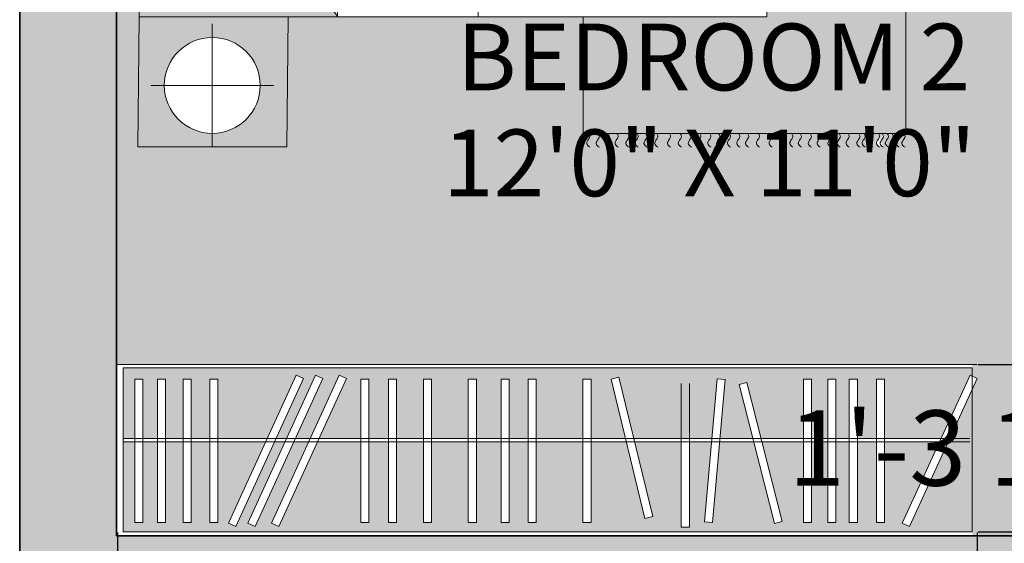
# Model space of a CAD drawing. Units: inches. Extents: x 1316 to 1777, y 813 to 1650.
# Tile 11 of 22: x 1377 to 1469, y 1434 to 1482. Entities that reach past the tile are written whole.
import ezdxf

# ---------------------------------------------------------------- set-up
doc = ezdxf.new("R2010")
doc.units = ezdxf.units.IN
doc.header["$MEASUREMENT"] = 0
for name, color, linetype, lineweight in [('A-ANNO-DIMS', 2, 'Continuous', 18), ('A-AREA-IDEN', 7, 'Continuous', 18), ('A-FURN-PATT', 23, 'Continuous', 13), ('A-WALL-PATT', 250, 'Continuous', 13), ('closet', 23, 'Continuous', 18), ('furniture', 23, 'Continuous', 18), ('walls', 250, 'Continuous', 35)]:
    doc.layers.add(name, color=color, linetype=linetype, lineweight=lineweight)
doc.layers.add('A-FLOR-PATT', color=254, linetype='Continuous', lineweight=13, true_color=0xfeeab9)
doc.styles.get("Standard").update_dxf_attribs({"font": 'arial.ttf'})
doc.dimstyles.get("Standard").update_dxf_attribs({"dimtxt": 7, "dimasz": 0.18, "dimexe": 0.18, "dimexo": 0.0625, "dimgap": 0.09, "dimtad": 0, "dimtih": 1, "dimtoh": 1, "dimzin": 0, "dimdsep": 46, "dimlunit": 3, "dimtxsty": 'Standard', "dimcen": 0.09, "dimadec": 0, "dimazin": 0, "dimtfac": 1, "dimtofl": 0, "dimtmove": 0, "dimatfit": 3, "dimfxl": 1, "dimtolj": 1, "dimtzin": 0, "dimarcsym": 0})

# ---------------------------------------------------------------- blocks, each defined once
blk = doc.blocks.new('CARPET')
at = {"layer": 'furniture'}
for p, q in [((-51.53, -98.11), (-51.53, -55.12)), ((-51.53, -55.12), (-41.27, -55.12)), ((36, -55.12), (51.55, -55.12)), ((51.55, -55.12), (51.55, -98.11)), ((51.55, -98.11), (-51.53, -98.11))]:
    blk.add_line(p, q, dxfattribs=at)
for points, knots in [([(-53.37, -55.99), (-53.22, -55.8), (-52.9, -55.41), (-52.34, -55.8), (-51.89, -56.08), (-51.65, -55.91), (-51.53, -55.83)], [0, 0, 0, 0, 0.653278, 1.290138, 1.740457, 2.114451, 2.114451, 2.114451, 2.114451]), ([(53.37, -55.99), (53.22, -55.8), (52.9, -55.41), (52.34, -55.8), (51.89, -56.08), (51.65, -55.91), (51.53, -55.83)], [0, 0, 0, 0, 0.653278, 1.290138, 1.740457, 2.114451, 2.114451, 2.114451, 2.114451]), ([(-53.37, -57.26), (-53.22, -57.07), (-52.9, -56.67), (-52.34, -57.07), (-51.89, -57.35), (-51.65, -57.17), (-51.53, -57.1)], [0, 0, 0, 0, 0.653278, 1.290138, 1.740457, 2.114451, 2.114451, 2.114451, 2.114451]), ([(53.37, -57.26), (53.22, -57.07), (52.9, -56.67), (52.34, -57.07), (51.89, -57.35), (51.65, -57.17), (51.53, -57.1)], [0, 0, 0, 0, 0.653278, 1.290138, 1.740457, 2.114451, 2.114451, 2.114451, 2.114451]), ([(-53.37, -58.59), (-53.22, -58.4), (-52.9, -58.01), (-52.34, -58.4), (-51.89, -58.68), (-51.65, -58.5), (-51.53, -58.43)], [0, 0, 0, 0, 0.653278, 1.290138, 1.740457, 2.114451, 2.114451, 2.114451, 2.114451]), ([(53.37, -58.59), (53.22, -58.4), (52.9, -58.01), (52.34, -58.4), (51.89, -58.68), (51.65, -58.5), (51.53, -58.43)], [0, 0, 0, 0, 0.653278, 1.290138, 1.740457, 2.114451, 2.114451, 2.114451, 2.114451]), ([(-53.37, -59.78), (-53.22, -59.58), (-52.9, -59.19), (-52.34, -59.58), (-51.89, -59.86), (-51.65, -59.69), (-51.53, -59.61)], [0, 0, 0, 0, 0.653278, 1.290138, 1.740457, 2.114451, 2.114451, 2.114451, 2.114451]), ([(53.37, -59.78), (53.22, -59.58), (52.9, -59.19), (52.34, -59.58), (51.89, -59.86), (51.65, -59.69), (51.53, -59.61)], [0, 0, 0, 0, 0.653278, 1.290138, 1.740457, 2.114451, 2.114451, 2.114451, 2.114451]), ([(-53.37, -61.22), (-53.22, -61.02), (-52.9, -60.63), (-52.34, -61.02), (-51.89, -61.3), (-51.65, -61.13), (-51.53, -61.05)], [0, 0, 0, 0, 0.653278, 1.290138, 1.740457, 2.114451, 2.114451, 2.114451, 2.114451]), ([(53.37, -61.22), (53.22, -61.02), (52.9, -60.63), (52.34, -61.02), (51.89, -61.3), (51.65, -61.13), (51.53, -61.05)], [0, 0, 0, 0, 0.653278, 1.290138, 1.740457, 2.114451, 2.114451, 2.114451, 2.114451]), ([(-53.37, -62.44), (-53.22, -62.25), (-52.9, -61.86), (-52.34, -62.25), (-51.89, -62.53), (-51.65, -62.36), (-51.53, -62.28)], [0, 0, 0, 0, 0.653278, 1.290138, 1.740457, 2.114451, 2.114451, 2.114451, 2.114451]), ([(53.37, -62.44), (53.22, -62.25), (52.9, -61.86), (52.34, -62.25), (51.89, -62.53), (51.65, -62.36), (51.53, -62.28)], [0, 0, 0, 0, 0.653278, 1.290138, 1.740457, 2.114451, 2.114451, 2.114451, 2.114451]), ([(-53.37, -63.63), (-53.22, -63.43), (-52.9, -63.04), (-52.34, -63.43), (-51.89, -63.72), (-51.65, -63.54), (-51.53, -63.46)], [0, 0, 0, 0, 0.653278, 1.290138, 1.740457, 2.114451, 2.114451, 2.114451, 2.114451]), ([(53.37, -63.63), (53.22, -63.43), (52.9, -63.04), (52.34, -63.43), (51.89, -63.72), (51.65, -63.54), (51.53, -63.46)], [0, 0, 0, 0, 0.653278, 1.290138, 1.740457, 2.114451, 2.114451, 2.114451, 2.114451]), ([(-53.37, -65.07), (-53.22, -64.87), (-52.9, -64.48), (-52.34, -64.87), (-51.89, -65.15), (-51.65, -64.98), (-51.53, -64.9)], [0, 0, 0, 0, 0.653278, 1.290138, 1.740457, 2.114451, 2.114451, 2.114451, 2.114451]), ([(53.37, -65.07), (53.22, -64.87), (52.9, -64.48), (52.34, -64.87), (51.89, -65.15), (51.65, -64.98), (51.53, -64.9)], [0, 0, 0, 0, 0.653278, 1.290138, 1.740457, 2.114451, 2.114451, 2.114451, 2.114451]), ([(-53.37, -66.76), (-53.22, -66.56), (-52.9, -66.17), (-52.34, -66.56), (-51.89, -66.84), (-51.65, -66.67), (-51.53, -66.59)], [0, 0, 0, 0, 0.653278, 1.290138, 1.740457, 2.114451, 2.114451, 2.114451, 2.114451]), ([(53.37, -66.76), (53.22, -66.56), (52.9, -66.17), (52.34, -66.56), (51.89, -66.84), (51.65, -66.67), (51.53, -66.59)], [0, 0, 0, 0, 0.653278, 1.290138, 1.740457, 2.114451, 2.114451, 2.114451, 2.114451]), ([(-53.37, -68.2), (-53.22, -68), (-52.9, -67.61), (-52.34, -68), (-51.89, -68.28), (-51.65, -68.11), (-51.53, -68.03)], [0, 0, 0, 0, 0.653278, 1.290138, 1.740457, 2.114451, 2.114451, 2.114451, 2.114451]), ([(53.37, -68.2), (53.22, -68), (52.9, -67.61), (52.34, -68), (51.89, -68.28), (51.65, -68.11), (51.53, -68.03)], [0, 0, 0, 0, 0.653278, 1.290138, 1.740457, 2.114451, 2.114451, 2.114451, 2.114451]), ([(-53.37, -69.53), (-53.22, -69.33), (-52.9, -68.94), (-52.34, -69.33), (-51.89, -69.61), (-51.65, -69.44), (-51.53, -69.36)], [0, 0, 0, 0, 0.653278, 1.290138, 1.740457, 2.114451, 2.114451, 2.114451, 2.114451]), ([(53.37, -69.53), (53.22, -69.33), (52.9, -68.94), (52.34, -69.33), (51.89, -69.61), (51.65, -69.44), (51.53, -69.36)], [0, 0, 0, 0, 0.653278, 1.290138, 1.740457, 2.114451, 2.114451, 2.114451, 2.114451]), ([(-53.37, -70.79), (-53.22, -70.6), (-52.9, -70.21), (-52.34, -70.6), (-51.89, -70.88), (-51.65, -70.7), (-51.53, -70.63)], [0, 0, 0, 0, 0.653278, 1.290138, 1.740457, 2.114451, 2.114451, 2.114451, 2.114451]), ([(53.37, -70.79), (53.22, -70.6), (52.9, -70.21), (52.34, -70.6), (51.89, -70.88), (51.65, -70.7), (51.53, -70.63)], [0, 0, 0, 0, 0.653278, 1.290138, 1.740457, 2.114451, 2.114451, 2.114451, 2.114451]), ([(-53.37, -72.12), (-53.22, -71.93), (-52.9, -71.54), (-52.34, -71.93), (-51.89, -72.21), (-51.65, -72.04), (-51.53, -71.96)], [0, 0, 0, 0, 0.653278, 1.290138, 1.740457, 2.114451, 2.114451, 2.114451, 2.114451]), ([(53.37, -72.12), (53.22, -71.93), (52.9, -71.54), (52.34, -71.93), (51.89, -72.21), (51.65, -72.04), (51.53, -71.96)], [0, 0, 0, 0, 0.653278, 1.290138, 1.740457, 2.114451, 2.114451, 2.114451, 2.114451]), ([(-53.37, -73.31), (-53.22, -73.11), (-52.9, -72.72), (-52.34, -73.11), (-51.89, -73.4), (-51.65, -73.22), (-51.53, -73.14)], [0, 0, 0, 0, 0.653278, 1.290138, 1.740457, 2.114451, 2.114451, 2.114451, 2.114451]), ([(53.37, -73.31), (53.22, -73.11), (52.9, -72.72), (52.34, -73.11), (51.89, -73.4), (51.65, -73.22), (51.53, -73.14)], [0, 0, 0, 0, 0.653278, 1.290138, 1.740457, 2.114451, 2.114451, 2.114451, 2.114451]), ([(-53.37, -74.75), (-53.22, -74.55), (-52.9, -74.16), (-52.34, -74.55), (-51.89, -74.83), (-51.65, -74.66), (-51.53, -74.58)], [0, 0, 0, 0, 0.653278, 1.290138, 1.740457, 2.114451, 2.114451, 2.114451, 2.114451]), ([(53.37, -74.75), (53.22, -74.55), (52.9, -74.16), (52.34, -74.55), (51.89, -74.83), (51.65, -74.66), (51.53, -74.58)], [0, 0, 0, 0, 0.653278, 1.290138, 1.740457, 2.114451, 2.114451, 2.114451, 2.114451]), ([(-53.37, -75.98), (-53.22, -75.78), (-52.9, -75.39), (-52.34, -75.78), (-51.89, -76.06), (-51.65, -75.89), (-51.53, -75.81)], [0, 0, 0, 0, 0.653278, 1.290138, 1.740457, 2.114451, 2.114451, 2.114451, 2.114451]), ([(53.37, -75.98), (53.22, -75.78), (52.9, -75.39), (52.34, -75.78), (51.89, -76.06), (51.65, -75.89), (51.53, -75.81)], [0, 0, 0, 0, 0.653278, 1.290138, 1.740457, 2.114451, 2.114451, 2.114451, 2.114451]), ([(-53.37, -77.16), (-53.22, -76.96), (-52.9, -76.57), (-52.34, -76.96), (-51.89, -77.25), (-51.65, -77.07), (-51.53, -76.99)], [0, 0, 0, 0, 0.653278, 1.290138, 1.740457, 2.114451, 2.114451, 2.114451, 2.114451]), ([(53.37, -77.16), (53.22, -76.96), (52.9, -76.57), (52.34, -76.96), (51.89, -77.25), (51.65, -77.07), (51.53, -76.99)], [0, 0, 0, 0, 0.653278, 1.290138, 1.740457, 2.114451, 2.114451, 2.114451, 2.114451]), ([(-53.37, -78.6), (-53.22, -78.4), (-52.9, -78.01), (-52.34, -78.4), (-51.89, -78.68), (-51.65, -78.51), (-51.53, -78.43)], [0, 0, 0, 0, 0.653278, 1.290138, 1.740457, 2.114451, 2.114451, 2.114451, 2.114451]), ([(53.37, -78.6), (53.22, -78.4), (52.9, -78.01), (52.34, -78.4), (51.89, -78.68), (51.65, -78.51), (51.53, -78.43)], [0, 0, 0, 0, 0.653278, 1.290138, 1.740457, 2.114451, 2.114451, 2.114451, 2.114451]), ([(-53.37, -80.29), (-53.22, -80.09), (-52.9, -79.7), (-52.34, -80.09), (-51.89, -80.37), (-51.65, -80.2), (-51.53, -80.12)], [0, 0, 0, 0, 0.653278, 1.290138, 1.740457, 2.114451, 2.114451, 2.114451, 2.114451]), ([(53.37, -80.29), (53.22, -80.09), (52.9, -79.7), (52.34, -80.09), (51.89, -80.37), (51.65, -80.2), (51.53, -80.12)], [0, 0, 0, 0, 0.653278, 1.290138, 1.740457, 2.114451, 2.114451, 2.114451, 2.114451]), ([(-53.37, -81.73), (-53.22, -81.53), (-52.9, -81.14), (-52.34, -81.53), (-51.89, -81.81), (-51.65, -81.64), (-51.53, -81.56)], [0, 0, 0, 0, 0.653278, 1.290138, 1.740457, 2.114451, 2.114451, 2.114451, 2.114451]), ([(53.37, -81.73), (53.22, -81.53), (52.9, -81.14), (52.34, -81.53), (51.89, -81.81), (51.65, -81.64), (51.53, -81.56)], [0, 0, 0, 0, 0.653278, 1.290138, 1.740457, 2.114451, 2.114451, 2.114451, 2.114451]), ([(-53.37, -83.06), (-53.22, -82.86), (-52.9, -82.47), (-52.34, -82.86), (-51.89, -83.14), (-51.65, -82.97), (-51.53, -82.89)], [0, 0, 0, 0, 0.653278, 1.290138, 1.740457, 2.114451, 2.114451, 2.114451, 2.114451]), ([(53.37, -83.06), (53.22, -82.86), (52.9, -82.47), (52.34, -82.86), (51.89, -83.14), (51.65, -82.97), (51.53, -82.89)], [0, 0, 0, 0, 0.653278, 1.290138, 1.740457, 2.114451, 2.114451, 2.114451, 2.114451]), ([(-53.37, -84.18), (-53.22, -83.99), (-52.9, -83.6), (-52.34, -83.99), (-51.89, -84.27), (-51.65, -84.09), (-51.53, -84.02)], [0, 0, 0, 0, 0.653278, 1.290138, 1.740457, 2.114451, 2.114451, 2.114451, 2.114451]), ([(53.37, -84.18), (53.22, -83.99), (52.9, -83.6), (52.34, -83.99), (51.89, -84.27), (51.65, -84.09), (51.53, -84.02)], [0, 0, 0, 0, 0.653278, 1.290138, 1.740457, 2.114451, 2.114451, 2.114451, 2.114451]), ([(-53.37, -85.51), (-53.22, -85.32), (-52.9, -84.93), (-52.34, -85.32), (-51.89, -85.6), (-51.65, -85.42), (-51.53, -85.35)], [0, 0, 0, 0, 0.653278, 1.290138, 1.740457, 2.114451, 2.114451, 2.114451, 2.114451]), ([(53.37, -85.51), (53.22, -85.32), (52.9, -84.93), (52.34, -85.32), (51.89, -85.6), (51.65, -85.42), (51.53, -85.35)], [0, 0, 0, 0, 0.653278, 1.290138, 1.740457, 2.114451, 2.114451, 2.114451, 2.114451]), ([(-53.37, -86.7), (-53.22, -86.5), (-52.9, -86.11), (-52.34, -86.5), (-51.89, -86.78), (-51.65, -86.61), (-51.53, -86.53)], [0, 0, 0, 0, 0.653278, 1.290138, 1.740457, 2.114451, 2.114451, 2.114451, 2.114451]), ([(53.37, -86.7), (53.22, -86.5), (52.9, -86.11), (52.34, -86.5), (51.89, -86.78), (51.65, -86.61), (51.53, -86.53)], [0, 0, 0, 0, 0.653278, 1.290138, 1.740457, 2.114451, 2.114451, 2.114451, 2.114451]), ([(-53.37, -88.14), (-53.22, -87.94), (-52.9, -87.55), (-52.34, -87.94), (-51.89, -88.22), (-51.65, -88.05), (-51.53, -87.97)], [0, 0, 0, 0, 0.653278, 1.290138, 1.740457, 2.114451, 2.114451, 2.114451, 2.114451]), ([(53.37, -88.14), (53.22, -87.94), (52.9, -87.55), (52.34, -87.94), (51.89, -88.22), (51.65, -88.05), (51.53, -87.97)], [0, 0, 0, 0, 0.653278, 1.290138, 1.740457, 2.114451, 2.114451, 2.114451, 2.114451]), ([(-53.37, -89.36), (-53.22, -89.17), (-52.9, -88.78), (-52.34, -89.17), (-51.89, -89.45), (-51.65, -89.28), (-51.53, -89.2)], [0, 0, 0, 0, 0.653278, 1.290138, 1.740457, 2.114451, 2.114451, 2.114451, 2.114451]), ([(53.37, -89.36), (53.22, -89.17), (52.9, -88.78), (52.34, -89.17), (51.89, -89.45), (51.65, -89.28), (51.53, -89.2)], [0, 0, 0, 0, 0.653278, 1.290138, 1.740457, 2.114451, 2.114451, 2.114451, 2.114451]), ([(-53.37, -90.55), (-53.22, -90.35), (-52.9, -89.96), (-52.34, -90.35), (-51.89, -90.64), (-51.65, -90.46), (-51.53, -90.38)], [0, 0, 0, 0, 0.653278, 1.290138, 1.740457, 2.114451, 2.114451, 2.114451, 2.114451]), ([(53.37, -90.55), (53.22, -90.35), (52.9, -89.96), (52.34, -90.35), (51.9, -90.63), (51.66, -90.47), (51.55, -90.4)], [0, 0, 0, 0, 0.653278, 1.290138, 1.740457, 2.0926, 2.0926, 2.0926, 2.0926]), ([(-53.37, -91.99), (-53.22, -91.79), (-52.9, -91.4), (-52.34, -91.79), (-51.89, -92.07), (-51.65, -91.9), (-51.53, -91.82)], [0, 0, 0, 0, 0.653278, 1.290138, 1.740457, 2.114451, 2.114451, 2.114451, 2.114451]), ([(53.37, -91.99), (53.22, -91.79), (52.9, -91.4), (52.34, -91.79), (51.9, -92.07), (51.66, -91.91), (51.55, -91.83)], [0, 0, 0, 0, 0.653278, 1.290138, 1.740457, 2.0926, 2.0926, 2.0926, 2.0926]), ([(-53.37, -92.69), (-53.22, -92.48), (-52.9, -92.08), (-52.35, -92.49), (-51.89, -92.77), (-51.65, -92.6), (-51.53, -92.52)], [0, 0, 0, 0, 0.663904, 1.307406, 1.757725, 2.131719, 2.131719, 2.131719, 2.131719]), ([(53.37, -92.69), (53.22, -92.49), (52.9, -92.09), (52.34, -92.49), (51.9, -92.77), (51.66, -92.61), (51.55, -92.53)], [0, 0, 0, 0, 0.656792, 1.295826, 1.746145, 2.098292, 2.098292, 2.098292, 2.098292]), ([(-53.37, -93.61), (-53.22, -93.42), (-52.9, -93.03), (-52.34, -93.42), (-51.89, -93.7), (-51.65, -93.52), (-51.53, -93.45)], [0, 0, 0, 0, 0.653278, 1.290138, 1.740457, 2.114451, 2.114451, 2.114451, 2.114451]), ([(-53.37, -94.55), (-53.22, -94.35), (-52.9, -93.96), (-52.34, -94.35), (-51.89, -94.63), (-51.65, -94.46), (-51.53, -94.38)], [0, 0, 0, 0, 0.653278, 1.290138, 1.740457, 2.114451, 2.114451, 2.114451, 2.114451]), ([(53.37, -93.66), (53.22, -93.46), (52.9, -93.07), (52.34, -93.46), (51.9, -93.74), (51.66, -93.58), (51.55, -93.5)], [0, 0, 0, 0, 0.653278, 1.290138, 1.740457, 2.0926, 2.0926, 2.0926, 2.0926]), ([(53.37, -94.59), (53.22, -94.4), (52.9, -94.01), (52.34, -94.4), (51.9, -94.68), (51.66, -94.51), (51.55, -94.44)], [0, 0, 0, 0, 0.653278, 1.290138, 1.740457, 2.0926, 2.0926, 2.0926, 2.0926]), ([(-53.37, -95.05), (-53.22, -94.85), (-52.9, -94.46), (-52.34, -94.85), (-51.89, -95.14), (-51.65, -94.96), (-51.53, -94.88)], [0, 0, 0, 0, 0.653278, 1.290138, 1.740457, 2.114451, 2.114451, 2.114451, 2.114451]), ([(-53.37, -95.73), (-53.22, -95.54), (-52.9, -95.15), (-52.34, -95.54), (-51.89, -95.82), (-51.65, -95.65), (-51.53, -95.57)], [0, 0, 0, 0, 0.653278, 1.290138, 1.740457, 2.114451, 2.114451, 2.114451, 2.114451]), ([(53.37, -95.78), (53.22, -95.58), (52.9, -95.19), (52.34, -95.58), (51.89, -95.86), (51.65, -95.69), (51.53, -95.61)], [0, 0, 0, 0, 0.653278, 1.290138, 1.740457, 2.114451, 2.114451, 2.114451, 2.114451]), ([(53.37, -95.1), (53.22, -94.9), (52.9, -94.51), (52.34, -94.9), (51.9, -95.18), (51.66, -95.02), (51.55, -94.94)], [0, 0, 0, 0, 0.653278, 1.290138, 1.740457, 2.0926, 2.0926, 2.0926, 2.0926]), ([(-53.37, -96.38), (-53.22, -96.18), (-52.9, -95.79), (-52.34, -96.18), (-51.89, -96.47), (-51.65, -96.29), (-51.53, -96.21)], [0, 0, 0, 0, 0.653278, 1.290138, 1.740457, 2.114451, 2.114451, 2.114451, 2.114451]), ([(-53.37, -97.17), (-53.22, -96.98), (-52.9, -96.59), (-52.34, -96.98), (-51.89, -97.26), (-51.65, -97.08), (-51.53, -97.01)], [0, 0, 0, 0, 0.653278, 1.290138, 1.740457, 2.114451, 2.114451, 2.114451, 2.114451]), ([(53.37, -96.43), (53.22, -96.23), (52.9, -95.84), (52.34, -96.23), (51.89, -96.51), (51.65, -96.34), (51.53, -96.26)], [0, 0, 0, 0, 0.653278, 1.290138, 1.740457, 2.114451, 2.114451, 2.114451, 2.114451]), ([(53.37, -97.22), (53.22, -97.02), (52.9, -96.63), (52.34, -97.02), (51.89, -97.3), (51.65, -97.13), (51.53, -97.05)], [0, 0, 0, 0, 0.653278, 1.290138, 1.740457, 2.114451, 2.114451, 2.114451, 2.114451]), ([(-53.37, -97.99), (-53.22, -97.79), (-52.9, -97.4), (-52.34, -97.79), (-51.89, -98.08), (-51.65, -97.9), (-51.53, -97.82)], [0, 0, 0, 0, 0.653278, 1.290138, 1.740457, 2.114451, 2.114451, 2.114451, 2.114451]), ([(53.37, -97.99), (53.22, -97.79), (52.9, -97.4), (52.34, -97.79), (51.89, -98.08), (51.65, -97.9), (51.53, -97.82)], [0, 0, 0, 0, 0.653278, 1.290138, 1.740457, 2.114451, 2.114451, 2.114451, 2.114451])]:
    blk.add_open_spline(points, degree=3, knots=knots, dxfattribs=at)
blk = doc.blocks.new('A$C58D270C6')
at = {"layer": 'furniture'}
for p, q in [((9.09, 124.13), (9.09, 108.87)), ((1.46, 116.5), (16.73, 116.5)), ((14.97, 94.84), (24.62, 107.92)), ((24.62, 94.93), (24.62, 107.92)), ((42.08, 108), (42.08, 36)), ((14.97, 94.93), (24.62, 94.93)), ((14.97, 94.84), (14.97, 36)), ((16.22, 94.93), (16.22, 36)), ((9.25, 36), (9.25, 20.74)), ((1.62, 28.37), (16.88, 28.37))]:
    blk.add_line(p, q, dxfattribs=at)
for points in [[(18.5, 108), (18.34, 124.13), (-0.16, 124.13), (0, 108)], [(0, 108), (77.91, 108), (77.91, 36), (0, 36)], [(4.09, 94.93), (14.97, 94.93), (14.97, 73.83), (4.09, 73.83)], [(4.09, 65.23), (14.97, 65.23), (14.97, 44.13), (4.09, 44.13)], [(18.65, 19.87), (18.5, 36), (0, 36), (0.16, 19.87)]]:
    blk.add_lwpolyline(points, close=True, dxfattribs=at)
for centre in [(9.09, 116.5), (9.25, 28.37)]:
    blk.add_circle(centre, 5.95, dxfattribs=at)
at = {"layer": 'furniture', "xscale": 0.9312884925094044, "yscale": 0.9312884925094044, "zscale": 0.9312884925094044, "rotation": 90}
blk.add_blockref('CARPET', (3.79, 74.47), dxfattribs=at)
blk = doc.blocks.new('closet')
at = {"layer": 'closet'}
for p, q in [((26.086, 8.254), (26.086, -5.103)), ((26.843, 8.254), (26.843, -5.103)), ((-0.712, -5.577), (5.592, 8.191)), ((-0.232, 7.394), (-0.232, -6.566)), ((6.268, 7.882), (-0.036, -5.886)), ((5.592, 8.191), (6.268, 7.882)), ((7.922, 7.842), (8.679, 7.842)), ((7.922, 7.842), (7.922, -5.515)), ((8.679, 7.842), (8.679, -5.515)), ((10.443, 7.842), (11.2, 7.842)), ((10.443, 7.842), (10.443, -5.515)), ((11.2, 7.842), (11.2, -5.515)), ((12.449, 7.842), (13.206, 7.842)), ((12.449, 7.842), (12.449, -5.515)), ((13.206, 7.842), (13.206, -5.515)), ((14.712, 7.842), (15.469, 7.842)), ((14.712, 7.842), (14.712, -5.515)), ((15.469, 7.842), (15.469, -5.515)), ((17.436, 7.748), (18.17, 7.935)), ((17.436, 7.748), (20.729, -5.196)), ((18.17, 7.935), (21.462, -5.009)), ((23.918, 7.842), (22.755, -5.464)), ((24.672, 7.776), (23.509, -5.53)), ((23.918, 7.842), (24.672, 7.776)), ((30.221, 7.465), (33.372, -5.515)), ((35.229, 7.842), (35.229, -5.515)), ((35.986, 7.842), (35.986, -5.515)), ((40.326, 7.842), (40.326, -5.515)), ((41.083, 7.842), (41.083, -5.515)), ((42.848, 7.842), (42.848, -5.515)), ((43.605, 7.842), (43.605, -5.515)), ((45.896, 7.842), (45.896, -5.515)), ((46.653, 7.842), (46.653, -5.515)), ((50.066, 7.842), (50.066, -5.515)), ((50.823, 7.842), (50.823, -5.515)), ((53.325, 7.842), (53.325, -5.515)), ((54.081, 7.842), (54.081, -5.515)), ((55.896, 7.842), (55.896, -5.515)), ((56.653, 7.842), (56.653, -5.515)), ((57.994, -5.577), (64.297, 8.191)), ((64.973, 7.882), (58.669, -5.886)), ((60.189, -5.577), (66.493, 8.191)), ((67.169, 7.882), (60.865, -5.886)), ((61.999, -5.577), (68.303, 8.191)), ((68.978, 7.882), (62.675, -5.886)), ((69.963, 7.842), (69.963, -5.515)), ((70.72, 7.842), (70.72, -5.515)), ((72.429, 7.842), (72.429, -5.515)), ((73.186, 7.842), (73.186, -5.515)), ((74.817, 7.842), (74.817, -5.515)), ((75.574, 7.842), (75.574, -5.515)), ((76.936, 7.842), (76.936, -5.515)), ((77.693, 7.842), (77.693, -5.515)), ((29.485, 7.286), (32.636, -5.694)), ((56.234, 0.335), (0, 0.335)), ((56.2, 0), (0, 0)), ((56.2, 0), (78.757, 0)), ((56.234, 0.335), (78.757, 0.335)), ((21.462, -5.009), (20.729, -5.196)), ((23.509, -5.53), (22.755, -5.464)), ((-0.036, -5.886), (-0.712, -5.577)), ((33.372, -5.515), (32.636, -5.694)), ((35.986, -5.515), (35.229, -5.515)), ((41.083, -5.515), (40.326, -5.515)), ((43.605, -5.515), (42.848, -5.515)), ((46.653, -5.515), (45.896, -5.515)), ((50.823, -5.515), (50.066, -5.515)), ((54.081, -5.515), (53.325, -5.515)), ((56.653, -5.515), (55.896, -5.515)), ((58.669, -5.886), (57.994, -5.577)), ((60.865, -5.886), (60.189, -5.577)), ((62.675, -5.886), (61.999, -5.577)), ((70.72, -5.515), (69.963, -5.515)), ((73.186, -5.515), (72.429, -5.515)), ((75.574, -5.515), (74.817, -5.515)), ((77.693, -5.515), (76.936, -5.515))]:
    blk.add_line(p, q, dxfattribs=at)
blk = doc.blocks.new('rotated closet')
at = {"layer": 'closet'}
for p, q in [((26.318, 0.86), (27.074, 0.86)), ((29.717, -0.108), (30.452, 0.071)), ((35.461, 0.448), (36.217, 0.448)), ((40.558, 0.448), (41.314, 0.448)), ((43.08, 0.448), (43.837, 0.448)), ((46.128, 0.448), (46.884, 0.448)), ((50.298, 0.448), (51.055, 0.448)), ((53.556, 0.448), (54.313, 0.448)), ((56.128, 0.448), (56.884, 0.448)), ((64.529, 0.797), (65.205, 0.488)), ((66.725, 0.797), (67.4, 0.488)), ((68.534, 0.797), (69.21, 0.488)), ((70.195, 0.448), (70.952, 0.448)), ((72.66, 0.448), (73.417, 0.448)), ((75.049, 0.448), (75.806, 0.448)), ((77.168, 0.448), (77.924, 0.448)), ((78.989, 0), (78.989, -13.96)), ((8.91, -12.909), (8.153, -12.909)), ((11.431, -12.909), (10.675, -12.909)), ((13.437, -12.909), (12.681, -12.909)), ((15.7, -12.909), (14.943, -12.909)), ((-0.456, -14.274), (79.544, -14.274)), ((0, -13.96), (78.989, -13.96))]:
    blk.add_line(p, q, dxfattribs=at)
blk.add_blockref('closet', (0.232, -7.394), dxfattribs=at)
blk = doc.blocks.new('WARDROBE-80')
for p, q in [((80, 15.567), (0, 15.567)), ((80, 15.567), (0, 15.567)), ((80, 15.567), (0, 15.567)), ((0.555, 15.252), (0.555, 0.442)), ((79.544, 15.252), (0.555, 15.252)), ((79.544, 15.252), (2.199, 15.252)), ((79.544, 0), (79.544, 15.252)), ((0.555, 0), (0.555, 0.442)), ((79.544, 0), (0.555, 0))]:
    blk.add_line(p, q)
at = {"rotation": 179.9999999959433}
blk.add_blockref('rotated closet', (79.544, 1.293), dxfattribs=at)
blk = doc.blocks.new('*D30')
at = {"layer": 'A-ANNO-DIMS', "color": 0, "lineweight": -2, "transparency": 16777216}
for p, q in [((1386.153, 1434.699), (1386.153, 1422.578)), ((1466.177, 1434.699), (1466.177, 1422.578)), ((1386.333, 1422.758), (1465.997, 1422.758)), ((1466.177, 1422.758), (1466.357, 1422.758))]:
    blk.add_line(p, q, dxfattribs=at)
at = {"layer": 'A-ANNO-DIMS', "color": 0, "transparency": 16777216}
for points in [[(1386.333, 1422.788), (1386.333, 1422.728), (1386.153, 1422.758)], [(1465.997, 1422.788), (1465.997, 1422.728), (1466.177, 1422.758)]]:
    blk.add_solid(points, dxfattribs=at)
at = {"layer": 'Defpoints', "color": 0, "transparency": 16777216}
for p in [(1386.153, 1434.762), (1466.177, 1434.762), (1466.177, 1422.758)]:
    blk.add_point(p, dxfattribs=at)
at = {"layer": 'A-ANNO-DIMS', "color": 0, "transparency": 16777216, "insert": (1518.078, 1422.758), "char_height": 7, "attachment_point": 5}
blk.add_mtext('\\A1;WARDROBE 6\'-8" TYP.', dxfattribs=at)
blk = doc.blocks.new('*D31')
at = {"layer": 'A-ANNO-DIMS', "color": 0, "lineweight": -2, "transparency": 16777216}
for p, q in [((1466.24, 1450.329), (1478.361, 1450.329)), ((1478.181, 1450.149), (1478.181, 1446.257)), ((1478.181, 1434.942), (1478.181, 1438.834)), ((1466.24, 1434.762), (1478.361, 1434.762))]:
    blk.add_line(p, q, dxfattribs=at)
at = {"layer": 'A-ANNO-DIMS', "color": 0, "transparency": 16777216}
for points in [[(1478.151, 1450.149), (1478.211, 1450.149), (1478.181, 1450.329)], [(1478.151, 1434.942), (1478.211, 1434.942), (1478.181, 1434.762)]]:
    blk.add_solid(points, dxfattribs=at)
at = {"layer": 'Defpoints', "color": 0, "transparency": 16777216}
for p in [(1466.177, 1450.329), (1478.181, 1450.329), (1466.177, 1434.762)]:
    blk.add_point(p, dxfattribs=at)
at = {"layer": 'A-ANNO-DIMS', "color": 0, "transparency": 16777216, "insert": (1478.181, 1442.545), "char_height": 7, "attachment_point": 5}
blk.add_mtext('\\A1;1\'-3 1/2" TYP.', dxfattribs=at)

msp = doc.modelspace()

# ---------------------------------------------------------------- hatches: boundary and pattern name
at = {"layer": 'A-FLOR-PATT'}
h = msp.add_hatch(color=256, dxfattribs=at)
h.dxf.hatch_style = 1
h.paths.add_polyline_path([(1704.173, 1566.369), (1574.845, 1566.369), (1574.845, 1434.369), (1704.173, 1434.369)])
h.paths.add_polyline_path([(1630.932, 1542.856), (1660.956, 1542.856), (1660.956, 1535.716), (1688.427, 1535.716), (1688.322, 1546.604), (1686.085, 1547.859), (1686.091, 1547.88), (1685.166, 1550.963), (1681.619, 1555.397), (1678.246, 1552.474), (1678.253, 1552.433), (1678.187, 1552.423), (1681.619, 1555.397), (1683.601, 1556.058), (1683.639, 1556.172), (1683.764, 1556.112), (1686.94, 1557.171), (1688.039, 1558.585), (1688.034, 1558.699), (1688.108, 1558.672), (1686.969, 1557.208), (1686.965, 1557.18), (1681.619, 1555.397), (1682.039, 1554.872), (1682.12, 1554.846), (1682.107, 1554.788), (1685.145, 1550.989), (1685.188, 1550.977), (1685.173, 1550.941), (1685.764, 1548.971), (1688.364, 1547.814), (1702.185, 1547.814), (1702.301, 1535.716), (1702.301, 1481.716), (1702.418, 1469.617), (1688.544, 1469.617), (1688.427, 1481.716), (1660.956, 1481.716), (1660.956, 1470.853), (1630.932, 1470.853)], flags=16)
h.paths.add_polyline_path([(1624.931, 1450.279), (1703.919, 1450.279), (1703.919, 1436.32), (1703.919, 1435.026), (1624.931, 1435.026), (1624.931, 1435.469)], flags=16)
h.paths.add_polyline_path([(1624.931, 1443.714), (1625.995, 1443.714), (1625.995, 1449.229), (1626.752, 1449.229), (1626.752, 1443.714), (1628.114, 1443.714), (1628.114, 1449.229), (1628.871, 1449.229), (1628.871, 1443.714), (1630.502, 1443.714), (1630.502, 1449.229), (1631.259, 1449.229), (1631.259, 1443.714), (1632.968, 1443.714), (1632.968, 1449.229), (1633.724, 1449.229), (1633.724, 1443.714), (1638.318, 1443.714), (1641.013, 1449.6), (1641.689, 1449.29), (1639.136, 1443.714), (1640.128, 1443.714), (1642.823, 1449.6), (1643.499, 1449.29), (1640.945, 1443.714), (1642.323, 1443.714), (1645.018, 1449.6), (1645.694, 1449.29), (1643.141, 1443.714), (1647.035, 1443.714), (1647.035, 1449.229), (1647.792, 1449.229), (1647.792, 1443.714), (1649.606, 1443.714), (1649.606, 1449.229), (1650.363, 1449.229), (1650.363, 1443.714), (1652.865, 1443.714), (1652.865, 1449.229), (1653.621, 1449.229), (1653.621, 1443.714), (1657.035, 1443.714), (1657.035, 1449.229), (1657.792, 1449.229), (1657.792, 1443.714), (1660.083, 1443.714), (1660.083, 1449.229), (1660.839, 1449.229), (1660.839, 1443.714), (1662.605, 1443.714), (1662.605, 1449.229), (1663.362, 1449.229), (1663.362, 1443.714), (1667.702, 1443.714), (1667.702, 1449.229), (1668.459, 1449.229), (1668.459, 1443.714), (1671.655, 1443.714), (1670.316, 1449.229), (1671.051, 1449.407), (1672.434, 1443.714), (1679.696, 1443.714), (1680.179, 1449.244), (1680.933, 1449.178), (1680.455, 1443.714), (1683.5, 1443.714), (1682.225, 1448.723), (1682.959, 1448.91), (1684.281, 1443.714), (1688.219, 1443.714), (1688.219, 1449.229), (1688.976, 1449.229), (1688.976, 1443.714), (1690.482, 1443.714), (1690.482, 1449.229), (1691.239, 1449.229), (1691.239, 1443.714), (1692.488, 1443.714), (1692.488, 1449.229), (1693.245, 1449.229), (1693.245, 1443.714), (1695.009, 1443.714), (1695.009, 1449.229), (1695.766, 1449.229), (1695.766, 1443.714), (1701.029, 1443.714), (1700.875, 1443.379), (1695.766, 1443.379), (1695.766, 1435.872), (1695.009, 1435.872), (1695.009, 1443.379), (1693.245, 1443.379), (1693.245, 1435.872), (1692.488, 1435.872), (1692.488, 1443.379), (1691.239, 1443.379), (1691.239, 1435.872), (1690.482, 1435.872), (1690.482, 1443.379), (1688.976, 1443.379), (1688.976, 1435.872), (1688.219, 1435.872), (1688.219, 1443.379), (1684.366, 1443.379), (1686.252, 1435.965), (1685.518, 1435.779), (1683.585, 1443.379), (1680.426, 1443.379), (1679.77, 1435.872), (1679.016, 1435.938), (1679.666, 1443.379), (1677.602, 1443.379), (1677.602, 1435.46), (1676.845, 1435.46), (1676.845, 1443.379), (1672.515, 1443.379), (1674.202, 1436.427), (1673.467, 1436.249), (1671.736, 1443.379), (1668.459, 1443.379), (1668.459, 1435.872), (1667.702, 1435.872), (1667.702, 1443.379), (1663.362, 1443.379), (1663.362, 1435.872), (1662.605, 1435.872), (1662.605, 1443.379), (1660.839, 1443.379), (1660.839, 1435.872), (1660.083, 1435.872), (1660.083, 1443.379), (1657.792, 1443.379), (1657.792, 1435.872), (1657.035, 1435.872), (1657.035, 1443.379), (1653.621, 1443.379), (1653.621, 1435.872), (1652.865, 1435.872), (1652.865, 1443.379), (1650.363, 1443.379), (1650.363, 1435.872), (1649.606, 1435.872), (1649.606, 1443.379), (1647.792, 1443.379), (1647.792, 1435.872), (1647.035, 1435.872), (1647.035, 1443.379), (1642.988, 1443.379), (1639.39, 1435.522), (1638.715, 1435.832), (1642.17, 1443.379), (1640.792, 1443.379), (1637.195, 1435.522), (1636.519, 1435.832), (1639.974, 1443.379), (1638.983, 1443.379), (1635.385, 1435.522), (1634.709, 1435.832), (1638.165, 1443.379), (1633.724, 1443.379), (1633.724, 1435.872), (1632.968, 1435.872), (1632.968, 1443.379), (1631.259, 1443.379), (1631.259, 1435.872), (1630.502, 1435.872), (1630.502, 1443.379), (1628.871, 1443.379), (1628.871, 1435.872), (1628.114, 1435.872), (1628.114, 1443.379), (1626.752, 1443.379), (1626.752, 1435.872), (1625.995, 1435.872), (1625.995, 1443.379), (1624.931, 1443.379)], flags=0)
h.paths.add_polyline_path([(1683.839, 1491.517), (1691.022, 1491.517), (1691.071, 1491.582), (1691.071, 1529.618), (1699.231, 1529.618), (1699.231, 1513.795), (1691.071, 1513.795), (1691.071, 1507.34), (1699.231, 1507.34), (1699.231, 1491.517), (1691.022, 1491.517), (1683.839, 1481.774)], flags=0)
h.paths.add_polyline_path([(1691.015, 1475.341, -1), (1699.947, 1475.341, -1)], flags=0)
h.paths.add_polyline_path([(1690.898, 1541.439, -1), (1699.83, 1541.439, -1)], flags=0)
h.paths.add_polyline_path([(1505.845, 1469.591), (1505.845, 1566.369), (1386.064, 1566.369), (1386.064, 1450.329), (1465.697, 1450.329), (1465.697, 1449.245), (1466.177, 1449.025), (1465.697, 1447.977), (1465.697, 1436.055), (1465.697, 1434.369), (1505.845, 1434.369), (1505.845, 1440.551), (1476.949, 1440.551), (1476.949, 1441.822), (1476.977, 1441.822, -0.400014)])
edge = h.paths.add_edge_path(flags=16)
edge.add_spline(control_points=[(1456.973, 1471.794), (1457.023, 1471.721), (1457.138, 1471.554), (1456.942, 1471.242), (1456.67, 1470.851), (1456.943, 1470.632), (1457.081, 1470.522)], knot_values=[0, 0, 0, 0, 0.352144, 0.802463, 1.439322, 2.0926, 2.0926, 2.0926, 2.0926], degree=3, periodic=0)
edge.add_spline(control_points=[(1457.325, 1471.794), (1457.375, 1471.721), (1457.49, 1471.554), (1457.294, 1471.242), (1457.022, 1470.851), (1457.295, 1470.632), (1457.433, 1470.522)], knot_values=[0, 0, 0, 0, 0.352144, 0.802463, 1.439322, 2.0926, 2.0926, 2.0926, 2.0926], degree=3, periodic=0)
edge = h.paths.add_edge_path(flags=16)
edge.add_line((1429.513, 1471.794), (1429.513, 1482.657))
edge.add_line((1429.513, 1482.657), (1402.042, 1482.657))
edge.add_line((1402.042, 1482.657), (1401.925, 1470.559))
edge.add_line((1401.925, 1470.559), (1388.051, 1470.559))
edge.add_line((1388.051, 1470.559), (1388.167, 1482.657))
edge.add_line((1388.167, 1482.657), (1388.167, 1536.657))
edge.add_line((1388.167, 1536.657), (1388.284, 1548.755))
edge.add_line((1388.284, 1548.755), (1402.158, 1548.755))
edge.add_line((1402.158, 1548.755), (1402.042, 1536.657))
edge.add_line((1402.042, 1536.657), (1429.513, 1536.657))
edge.add_line((1429.513, 1536.657), (1429.513, 1543.797))
edge.add_line((1429.513, 1543.797), (1456.932, 1543.797))
edge.add_spline(control_points=[(1456.932, 1543.797), (1456.987, 1543.874), (1457.108, 1544.044), (1456.911, 1544.361), (1456.638, 1544.752), (1456.911, 1544.971), (1457.049, 1545.082)], knot_values=[0, 0, 0, 0, 0.373994, 0.824314, 1.461173, 2.114451, 2.114451, 2.114451, 2.114451], degree=3, periodic=0)
edge.add_spline(control_points=[(1457.401, 1545.082), (1457.263, 1544.971), (1456.99, 1544.752), (1457.263, 1544.361), (1457.46, 1544.044), (1457.339, 1543.874), (1457.284, 1543.797)], knot_values=[0, 0, 0, 0, 0.653278, 1.290138, 1.740457, 2.114451, 2.114451, 2.114451, 2.114451], degree=3, periodic=0)
edge.add_line((1457.284, 1543.797), (1459.536, 1543.797))
edge.add_line((1459.536, 1543.797), (1459.536, 1471.794))
edge.add_line((1459.536, 1471.794), (1429.513, 1471.794))
h.paths.add_polyline_path([(1406.63, 1482.715), (1399.446, 1492.458), (1399.398, 1492.458), (1391.238, 1492.458), (1391.238, 1508.281), (1399.398, 1508.281), (1399.398, 1514.736), (1391.238, 1514.736), (1391.238, 1530.559), (1399.398, 1530.559), (1399.398, 1492.524), (1399.446, 1492.458), (1406.63, 1492.458)], flags=0)
h.paths.add_polyline_path([(1399.454, 1476.282, -1), (1390.522, 1476.282, -1)], flags=0)
h.paths.add_polyline_path([(1390.638, 1542.38, -1), (1399.571, 1542.38, -1)], flags=0)
h.paths.add_polyline_path([(1487.293, 1548.286), (1487.08, 1548.252), (1487.104, 1547.964)], flags=16)
h.paths.add_polyline_path([(1491.493, 1552.843), (1490.887, 1552.654), (1490.949, 1552.372)], flags=16)
h.paths.add_polyline_path([(1489.966, 1554.409), (1489.859, 1554.561), (1489.718, 1554.445)], flags=16)
h.paths.add_polyline_path([(1497.301, 1546.483), (1497.294, 1546.462), (1497.309, 1546.453)], flags=16)
h.paths.add_polyline_path([(1496.386, 1549.553), (1492.828, 1554), (1492.655, 1554.939), (1492.454, 1555.029), (1492.589, 1555.296), (1491.806, 1559.547), (1491.869, 1559.506), (1491.824, 1559.451), (1492.828, 1554), (1494.81, 1554.661), (1494.848, 1554.774), (1494.973, 1554.715), (1496.01, 1555.061), (1496.078, 1555.314), (1496.341, 1555.171), (1498.15, 1555.774), (1499.249, 1557.187), (1499.243, 1557.301), (1499.317, 1557.275), (1498.179, 1555.811), (1498.174, 1555.782), (1492.828, 1554), (1493.249, 1553.474), (1493.33, 1553.449), (1493.316, 1553.39), (1495.203, 1551.032), (1495.702, 1550.957), (1495.574, 1550.568), (1496.354, 1549.592), (1496.397, 1549.58)], flags=16)
h.paths.add_polyline_path([(1486.021, 1555.224), (1485.958, 1555.549), (1483.595, 1557.912), (1483.28, 1557.859), (1483.243, 1558.264), (1486.27, 1555.237)], flags=16)
h.paths.add_polyline_path([(1505.845, 1469.591, 0.400014), (1476.977, 1441.822), (1505.845, 1441.822)], flags=17)
at = {"layer": 'A-FURN-PATT'}
h = msp.add_hatch(color=256, dxfattribs=at)
h.dxf.hatch_style = 1
h.paths.add_polyline_path([(1429.479, 1448.964), (1430.236, 1448.964), (1430.236, 1443.449), (1433.432, 1443.449), (1432.094, 1448.964), (1432.829, 1449.142), (1434.211, 1443.449), (1441.473, 1443.449), (1441.957, 1448.979), (1442.711, 1448.913), (1442.233, 1443.449), (1445.277, 1443.449), (1444.003, 1448.458), (1444.736, 1448.645), (1446.058, 1443.449), (1449.997, 1443.449), (1449.997, 1448.964), (1450.753, 1448.964), (1450.753, 1443.449), (1452.259, 1443.449), (1452.259, 1448.964), (1453.016, 1448.964), (1453.016, 1443.449), (1454.266, 1443.449), (1454.266, 1448.964), (1455.022, 1448.964), (1455.022, 1443.449), (1456.787, 1443.449), (1456.787, 1448.964), (1457.544, 1448.964), (1457.544, 1443.449), (1462.806, 1443.449), (1465.501, 1449.335), (1465.697, 1449.245), (1465.697, 1450.014), (1386.708, 1450.014), (1386.708, 1443.449), (1387.773, 1443.449), (1387.773, 1448.964), (1388.529, 1448.964), (1388.529, 1443.449), (1389.891, 1443.449), (1389.891, 1448.964), (1390.648, 1448.964), (1390.648, 1443.449), (1392.28, 1443.449), (1392.28, 1448.964), (1393.037, 1448.964), (1393.037, 1443.449), (1394.745, 1443.449), (1394.745, 1448.964), (1395.502, 1448.964), (1395.502, 1443.449), (1400.096, 1443.449), (1402.791, 1449.335), (1403.467, 1449.025), (1400.913, 1443.449), (1401.905, 1443.449), (1404.6, 1449.335), (1405.276, 1449.025), (1402.723, 1443.449), (1404.101, 1443.449), (1406.796, 1449.335), (1407.472, 1449.025), (1404.918, 1443.449), (1408.812, 1443.449), (1408.812, 1448.964), (1409.569, 1448.964), (1409.569, 1443.449), (1411.384, 1443.449), (1411.384, 1448.964), (1412.141, 1448.964), (1412.141, 1443.449), (1414.642, 1443.449), (1414.642, 1448.964), (1415.399, 1448.964), (1415.399, 1443.449), (1418.813, 1443.449), (1418.813, 1448.964), (1419.569, 1448.964), (1419.569, 1443.449), (1421.86, 1443.449), (1421.86, 1448.964), (1422.617, 1448.964), (1422.617, 1443.449), (1424.382, 1443.449), (1424.382, 1448.964), (1425.139, 1448.964), (1425.139, 1443.449), (1429.479, 1443.449)])
h.paths.add_polyline_path([(1429.479, 1443.114), (1425.139, 1443.114), (1425.139, 1435.607), (1424.382, 1435.607), (1424.382, 1443.114), (1422.617, 1443.114), (1422.617, 1435.607), (1421.86, 1435.607), (1421.86, 1443.114), (1419.569, 1443.114), (1419.569, 1435.607), (1418.813, 1435.607), (1418.813, 1443.114), (1415.399, 1443.114), (1415.399, 1435.607), (1414.642, 1435.607), (1414.642, 1443.114), (1412.141, 1443.114), (1412.141, 1435.607), (1411.384, 1435.607), (1411.384, 1443.114), (1409.569, 1443.114), (1409.569, 1435.607), (1408.812, 1435.607), (1408.812, 1443.114), (1404.765, 1443.114), (1401.168, 1435.258), (1400.492, 1435.567), (1403.948, 1443.114), (1402.57, 1443.114), (1398.972, 1435.258), (1398.296, 1435.567), (1401.752, 1443.114), (1400.76, 1443.114), (1397.163, 1435.258), (1396.487, 1435.567), (1399.943, 1443.114), (1395.502, 1443.114), (1395.502, 1435.607), (1394.745, 1435.607), (1394.745, 1443.114), (1393.037, 1443.114), (1393.037, 1435.607), (1392.28, 1435.607), (1392.28, 1443.114), (1390.648, 1443.114), (1390.648, 1435.607), (1389.891, 1435.607), (1389.891, 1443.114), (1388.529, 1443.114), (1388.529, 1435.607), (1387.773, 1435.607), (1387.773, 1443.114), (1386.708, 1443.114), (1386.708, 1436.055), (1386.708, 1435.204), (1386.708, 1434.762), (1465.697, 1434.762), (1465.697, 1447.977), (1459.873, 1435.258), (1459.197, 1435.567), (1462.653, 1443.114), (1457.544, 1443.114), (1457.544, 1435.607), (1456.787, 1435.607), (1456.787, 1443.114), (1455.022, 1443.114), (1455.022, 1435.607), (1454.266, 1435.607), (1454.266, 1443.114), (1453.016, 1443.114), (1453.016, 1435.607), (1452.259, 1435.607), (1452.259, 1443.114), (1450.753, 1443.114), (1450.753, 1435.607), (1449.997, 1435.607), (1449.997, 1443.114), (1446.143, 1443.114), (1448.029, 1435.7), (1447.296, 1435.514), (1445.362, 1443.114), (1442.204, 1443.114), (1441.547, 1435.607), (1440.793, 1435.673), (1441.444, 1443.114), (1439.379, 1443.114), (1439.379, 1435.195), (1438.623, 1435.195), (1438.623, 1443.114), (1434.292, 1443.114), (1435.98, 1436.163), (1435.245, 1435.984), (1433.514, 1443.114), (1430.236, 1443.114), (1430.236, 1435.607), (1429.479, 1435.607)])
h.paths.add_polyline_path([(1402.042, 1482.657), (1388.167, 1482.657), (1388.051, 1470.559), (1394.988, 1470.559), (1394.988, 1471.816, -0.414214), (1390.522, 1476.282, -1), (1399.454, 1476.282, -0.414214), (1394.988, 1471.816), (1394.988, 1470.559), (1401.925, 1470.559)])
h.paths.add_polyline_path([(1399.398, 1514.736), (1391.238, 1514.736), (1391.238, 1530.559), (1399.398, 1530.559), (1399.398, 1536.657), (1388.167, 1536.657), (1388.167, 1482.657), (1406.63, 1482.657), (1406.63, 1482.715), (1399.446, 1492.458), (1391.238, 1492.458), (1391.238, 1508.281), (1399.398, 1508.281)])
h.paths.add_polyline_path([(1399.571, 1542.38, -0.414214), (1395.105, 1537.914), (1395.105, 1536.657), (1402.042, 1536.657), (1402.158, 1548.755), (1388.284, 1548.755), (1388.167, 1536.657), (1395.105, 1536.657), (1395.105, 1537.914, -0.414214), (1390.638, 1542.38, -1)])
h = msp.add_hatch(color=256, dxfattribs=at)
h.dxf.hatch_style = 1
h.paths.add_polyline_path([(1399.398, 1508.281), (1391.238, 1508.281), (1391.238, 1492.458), (1399.398, 1492.458)])
h.paths.add_polyline_path([(1399.398, 1530.559), (1391.238, 1530.559), (1391.238, 1514.736), (1399.398, 1514.736)])
h.paths.add_polyline_path([(1459.536, 1543.797), (1429.513, 1543.797), (1429.513, 1536.657), (1446.596, 1536.657), (1446.596, 1482.657), (1429.513, 1482.657), (1429.513, 1471.794), (1459.536, 1471.794)])
at = {"layer": 'A-WALL-PATT'}
h = msp.add_hatch(color=256, dxfattribs=at)
h.dxf.hatch_style = 1
h.paths.add_polyline_path([(1713.173, 1281.369), (1656.173, 1281.369), (1656.173, 1298.258), (1651.673, 1298.258), (1651.673, 1281.369), (1567.673, 1281.369), (1567.673, 1266.995), (1572.173, 1266.995), (1572.173, 1276.869), (1704.173, 1276.869), (1704.173, 1132.869), (1608.64, 1132.869), (1608.64, 1123.869), (1704.173, 1123.869), (1704.173, 1040.173), (1652.869, 1040.173), (1652.869, 1031.173), (1713.173, 1031.173), (1713.173, 1040.173)])
h.paths.add_polyline_path([(1572.173, 1237.955), (1567.673, 1237.955), (1567.673, 1123.869), (1583.146, 1123.869), (1583.146, 1132.869), (1572.173, 1132.869)], flags=17)
h.paths.add_polyline_path([(1510.345, 1566.369), (1524.171, 1566.369), (1524.171, 1571.985), (1524.171, 1575.369), (1445.955, 1575.369), (1445.955, 1566.369), (1505.845, 1566.369), (1505.845, 1469.591), (1510.345, 1469.591), (1510.345, 1471.869), (1529.081, 1471.869), (1529.081, 1476.369), (1510.345, 1476.369)])
h.paths.add_polyline_path([(1609.722, 1575.369), (1545.119, 1575.369), (1545.119, 1566.369), (1570.345, 1566.369), (1570.345, 1476.369), (1562.477, 1476.369), (1562.477, 1471.869), (1570.345, 1471.869), (1570.345, 1469.591), (1574.845, 1469.591), (1574.845, 1566.369), (1609.722, 1566.369)])
h.paths.add_polyline_path([(1713.173, 1575.369), (1655.233, 1575.369), (1655.233, 1566.369), (1704.173, 1566.369), (1704.173, 1434.369), (1574.845, 1434.369), (1574.845, 1440.551), (1574.701, 1440.551), (1570.345, 1440.551), (1570.345, 1429.869), (1597.673, 1429.869), (1597.673, 1408.281), (1602.173, 1408.281), (1602.173, 1429.869), (1704.173, 1429.869), (1704.173, 1410.704), (1707.375, 1410.704), (1713.173, 1410.704)])
h.paths.add_polyline_path([(1713.173, 1383.676), (1704.173, 1383.676), (1704.173, 1369.869), (1602.173, 1369.869), (1602.173, 1379.241), (1597.673, 1379.241), (1597.673, 1365.369), (1713.173, 1365.369)])
h.paths.add_polyline_path([(1444.564, 1429.869), (1510.345, 1429.869), (1510.345, 1440.551), (1505.845, 1440.551), (1505.845, 1434.369), (1386.064, 1434.369), (1386.064, 1566.369), (1400.445, 1566.369), (1400.445, 1575.369), (1377.064, 1575.369), (1377.064, 1412.813), (1380.509, 1412.813), (1386.064, 1412.813), (1386.064, 1429.869), (1440.064, 1429.869), (1440.064, 1401.229), (1444.564, 1401.229)])
h.paths.add_polyline_path([(1444.564, 1372.189), (1440.064, 1372.189), (1440.064, 1369.869), (1386.064, 1369.869), (1386.064, 1378.758), (1377.064, 1378.758), (1377.064, 1349.201), (1381.118, 1349.201), (1386.064, 1349.201), (1386.064, 1365.369), (1440.064, 1365.369), (1440.064, 1322.882), (1444.564, 1322.882)])
h.paths.add_polyline_path([(1510.564, 1295.094), (1506.064, 1295.094), (1506.064, 1245.369), (1386.064, 1245.369), (1386.064, 1272.582), (1377.064, 1272.582), (1377.064, 1212.905), (1380.1, 1212.905), (1386.064, 1212.905), (1386.064, 1240.869), (1510.564, 1240.869)])
h.paths.add_polyline_path([(1386.064, 1163.761), (1377.064, 1163.761), (1377.064, 1063.869), (1419.363, 1063.869), (1419.363, 1072.869), (1386.064, 1072.869)])
h.paths.add_polyline_path([(1510.564, 1072.869), (1469.381, 1072.869), (1469.381, 1063.869), (1501.564, 1063.869), (1501.564, 1033.023), (1501.564, 1031.173), (1540.829, 1031.173), (1540.829, 1036.182, -0.029954), (1541.068, 1040.173), (1510.564, 1040.173)])
h.paths.add_polyline_path([(1607.369, 1040.173), (1574.225, 1040.173), (1574.225, 1036.182), (1574.225, 1031.173), (1607.369, 1031.173)], flags=17)
h.paths.add_polyline_path([(1637.054, 1040.173), (1624.706, 1040.173), (1624.706, 1031.173), (1637.054, 1031.173)], flags=17)

# ---------------------------------------------------------------- linework, layer by layer
at = {"layer": 'walls'}
for p, q in [((1377.064, 1575.369), (1377.064, 953.689)), ((1386.064, 1566.369), (1386.064, 1434.369)), ((1386.064, 1434.369), (1505.845, 1434.369))]:
    msp.add_line(p, q, dxfattribs=at)

# ---------------------------------------------------------------- block references
at = {"layer": 'closet'}
msp.add_blockref('WARDROBE-80', (1386.153, 1434.762), dxfattribs=at)
at = {"layer": 'furniture', "xscale": -0.7500000390647866, "yscale": 0.7500000390647866, "zscale": 0.7500000390647866, "rotation": 180}
msp.add_blockref('A$C58D270C6', (1388.167, 1563.657), dxfattribs=at)

# ---------------------------------------------------------------- texts
at = {"layer": 'A-AREA-IDEN'}
for s, height, p in [('BEDROOM 2', 6.206, (1417.736, 1475.826)), ('12\'0" X 11\'0"', 6.20603, (1416.467, 1465.977))]:
    msp.add_text(s, height=height, dxfattribs=at).set_placement(p)

# ---------------------------------------------------------------- dimensions: what is measured, and where the dimension line sits
at = {"layer": 'A-ANNO-DIMS'}
dim = msp.add_linear_dim(base=(1478.181, 1450.329), p1=(1466.177, 1434.762), p2=(1466.177, 1450.329), angle=90, text='<> TYP.', dimstyle='Standard', override={"dimdec": 1, "dimlfac": 1, "dimrnd": 0, "dimzin": 1, "dimdsep": 46, "dimlunit": 4, "dimfrac": 2}, dxfattribs=at)
dim.commit()
dim.dimension.update_dxf_attribs({"geometry": '*D31', "text_midpoint": (1478.181, 1442.545)})
dim = msp.add_linear_dim(base=(1466.177, 1422.758), p1=(1386.153, 1434.762), p2=(1466.177, 1434.762), text='WARDROBE <> TYP.', dimstyle='Standard', override={"dimdec": 1, "dimlfac": 1, "dimrnd": 0, "dimzin": 1, "dimdsep": 46, "dimlunit": 4, "dimfrac": 2}, dxfattribs=at)
dim.commit()
dim.dimension.update_dxf_attribs({"geometry": '*D30', "text_midpoint": (1518.078, 1422.758)})

doc.saveas('drawing.dxf')
